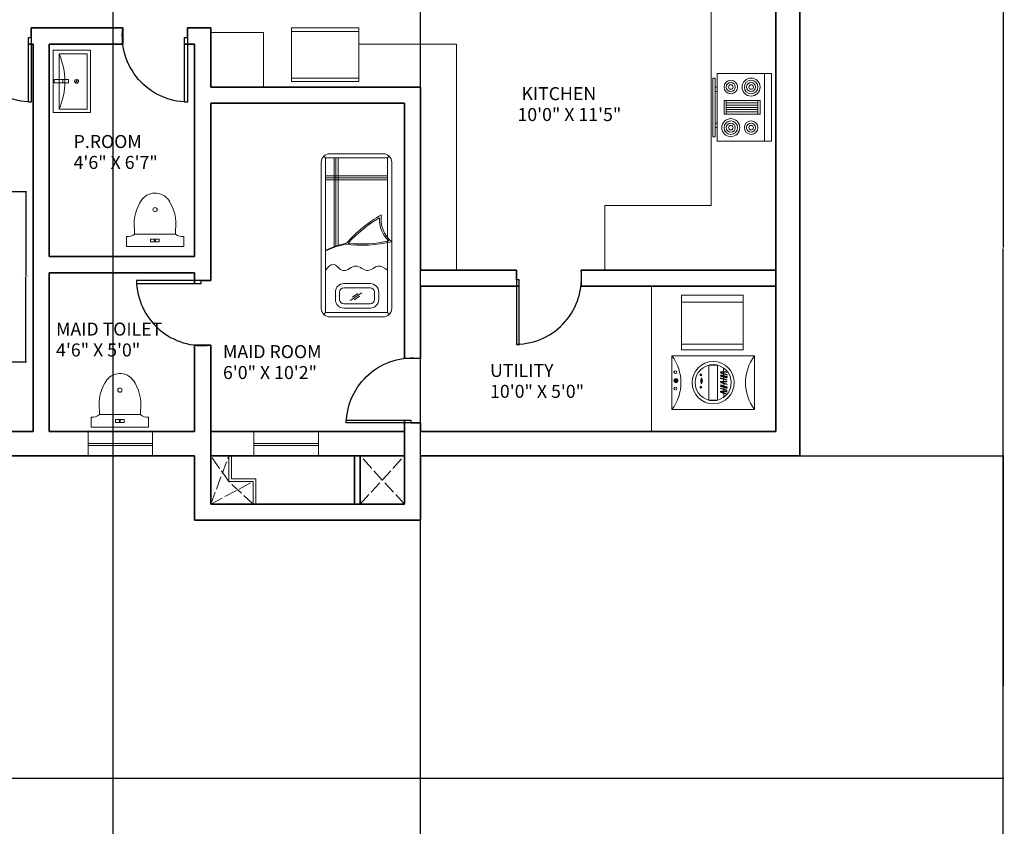
# Model space of a CAD drawing. Units: inches. Extents: x -61 to 1599, y -1316 to 257.
# Tile 195 of 204: x 1233 to 1599, y -579 to -279. Entities that reach past the tile are written whole.
import ezdxf

# ---------------------------------------------------------------- set-up
doc = ezdxf.new("R2010")
doc.units = ezdxf.units.IN
doc.header["$MEASUREMENT"] = 0
doc.linetypes.add('ACAD_ISO02W100', pattern=[15, 12, -3])
for name, color, linetype, lineweight in [('A-ANNO-DIMS', 2, 'Continuous', 18), ('A-AREA-IDEN', 1, 'Continuous', 18), ('A-EQPM', 9, 'Continuous', 18), ('A-FLOR-CASE', 8, 'Continuous', 18), ('A-FLOR-FIXT', 8, 'Continuous', 18), ('A-FLOR-OPEN-HIDN', 8, 'ACAD_ISO02W100', 13), ('A-WALL-JAMB', 4, 'ACAD_ISO02W100', 25), ('DOORS', 2, 'Continuous', 25), ('FURNITURE', 83, 'Continuous', 18), ('WALLS', 4, 'Continuous', 35), ('WINDOWS', 220, 'Continuous', 18)]:
    doc.layers.add(name, color=color, linetype=linetype, lineweight=lineweight)
doc.styles.get("Standard").update_dxf_attribs({"font": 'arial.ttf'})
doc.dimstyles.get("Standard").update_dxf_attribs({"dimtxt": 0.18, "dimasz": 0.18, "dimexe": 0.18, "dimexo": 0.0625, "dimgap": 0.09, "dimtad": 0, "dimtih": 1, "dimtoh": 1, "dimdec": 0, "dimzin": 0, "dimdsep": 46, "dimlunit": 3, "dimtxsty": 'Standard', "dimcen": 0.09, "dimadec": 0, "dimazin": 0, "dimtfac": 1, "dimtdec": 0, "dimtofl": 0, "dimtmove": 0, "dimatfit": 3, "dimfxl": 1, "dimtolj": 1, "dimtzin": 0, "dimarcsym": 0})

# ---------------------------------------------------------------- blocks, each defined once
blk = doc.blocks.new('Range-Oven - 30 in top')
for p, q in [((0, -3), (30, -3)), ((12, -6), (18, -6)), ((13, -20), (13, -6)), ((14, -6), (14, -20)), ((15, -20), (15, -6)), ((16, -6), (16, -20)), ((17, -20), (17, -6)), ((18, -20), (12, -20)), ((6, -24), (6, -25)), ((8, -25), (8, -24)), ((22, -25), (22, -24)), ((24, -24), (24, -25))]:
    blk.add_line(p, q)
for points in [[(0, -24), (0, 0), (30, 0), (30, -24)], [(12, -21), (12, -5), (18, -5), (18, -21)], [(2, -26), (2, -25), (28, -25), (28, -26)]]:
    blk.add_lwpolyline(points, close=True)
for centre, radius in [((6, -9), 4), ((6, -9), 3), ((6, -9), 2), ((6, -9), 1), ((24, -9), 3), ((24, -9), 2), ((24, -9), 1), ((6, -18), 3), ((6, -18), 2), ((6, -18), 1), ((24, -18), 4), ((24, -18), 3), ((24, -18), 2), ((24, -18), 1)]:
    blk.add_circle(centre, radius)
blk = doc.blocks.new('DOOR-SWING-24')
blk.add_line((0, 0), (0, 3.6))
blk.add_lwpolyline([(0, 0), (0, -24), (1.05, -24), (1.05, 0)], close=True)
blk.add_arc((-0.44, 0.62), 24.62, 271.0259, 6.9559)
blk = doc.blocks.new('WIN-24IN')
for p, q in [((0, 4.5), (0, 9)), ((0, 9), (0, 0)), ((24, 9), (24, 0)), ((0, 5.19), (24, 5.19)), ((0, 4.5), (24, 4.5))]:
    blk.add_line(p, q)
blk = doc.blocks.new('WC-FLOOR-MOUNT')
for p, q in [((0, 0), (0, 3.75)), ((3.02, 4.69), (3.02, 6.17)), ((3.02, 4.69), (18.31, 4.69)), ((18.31, 4.69), (18.31, 6.17)), ((21.33, 0), (21.33, 3.75)), ((0, 0), (21.33, 0))]:
    blk.add_line(p, q)
blk.add_lwpolyline([(12.24, 1.73), (8.96, 1.73), (8.96, 2.81), (12.24, 2.81)], close=True)
for centre, radius in [((10.67, 13.73), 0.792), ((10.6, 2.27), 0.208)]:
    blk.add_circle(centre, radius)
for centre, radius, start, end in [((10.67, 13.73), 6.18, 27.6844, 141.4697), ((19.05, 8.26), 16.17, 144.824, 187.4232), ((2.28, 8.26), 16.17, 352.5768, 35.176), ((0.56, 7.25), 3.55, 260.8586, 313.6993), ((20.77, 7.25), 3.55, 226.3007, 279.1414)]:
    blk.add_arc(centre, radius, start, end)
blk = doc.blocks.new('LAVATORY-WALL-2')
blk.add_line((3.67, 10.96), (3.67, 12.19))
for points in [[(0, 23.07), (13.87, 23.07), (13.87, 0), (0, 0)], [(12.66, 21.73), (12.66, 1.19), (2.2, 1.19), (2.2, 21.73)], [(5.78, 12.19), (5.78, 10.96), (0.4, 10.96), (0.4, 12.19)]]:
    blk.add_lwpolyline(points, close=True)
for radius in [0.74, 0.233]:
    blk.add_circle((8.7, 11.57), radius)
blk.add_arc((-20.86, 11.46), 25.25, 335.9939, 24.0061)
blk = doc.blocks.new('WASHING-MACHINE')
for p, q in [((19.24, 4.47), (19.22, 15.41)), ((0.96, 11.16), (1.13, 11)), ((1.49, 11.38), (1.49, 11.15)), ((2.02, 11.15), (1.86, 10.99)), ((11, 9.47), (11, 11.68)), ((0.98, 10.64), (0.75, 10.64)), ((1.12, 10.28), (0.96, 10.12)), ((1.49, 10.12), (1.49, 9.89)), ((1.86, 10.28), (2.02, 10.12)), ((2.23, 10.64), (2, 10.64))]:
    blk.add_line(p, q)
for points in [[(30.68, 0), (0, 0), (0, 19.87), (30.68, 19.87)], [(16.98, 3.42), (13.7, 3.42), (13.7, 16.45), (16.98, 16.45)], [(20.43, 13.78), (18.01, 13.78), (18.01, 13.95), (20.43, 13.95)], [(18.09, 12.45), (20.41, 11.74), (20.35, 11.57), (18.04, 12.29)], [(18.1, 11.71), (20.41, 10.99), (20.36, 10.83), (18.05, 11.54)], [(18.21, 13.64), (20.52, 12.92), (20.47, 12.76), (18.16, 13.47)], [(18.22, 12.89), (20.53, 12.18), (20.48, 12.01), (18.17, 12.73)], [(20.44, 10.23), (18.02, 10.23), (18.02, 10.4), (20.44, 10.4)], [(18.1, 8.63), (20.42, 7.91), (20.37, 7.75), (18.05, 8.46)], [(18.11, 7.88), (20.42, 7.17), (20.37, 7), (18.06, 7.72)], [(18.22, 10.09), (20.53, 9.38), (20.48, 9.21), (18.17, 9.92)], [(18.23, 9.07), (20.54, 8.36), (20.49, 8.19), (18.18, 8.91)], [(20.45, 6.56), (18.03, 6.56), (18.03, 6.73), (20.45, 6.73)], [(18.23, 6.42), (20.54, 5.7), (20.49, 5.54), (18.18, 6.25)]]:
    blk.add_lwpolyline(points, close=True)
for centre, radius in [((15.34, 9.94), 7.85), ((15.34, 9.94), 7.85), ((15.34, 9.94), 6.71), ((1.28, 13.83), 0.526), ((1.49, 10.64), 0.742), ((1.49, 10.64), 0.513), ((10.77, 12.86), 0.381), ((10.77, 12.86), 0.289), ((1.28, 7.75), 0.526), ((1.49, 10.64), 0.178), ((1.49, 10.64), 0.07), ((10.77, 8.29), 0.381), ((10.77, 8.29), 0.289)]:
    blk.add_circle(centre, radius)
for centre, radius, start, end in [((-13.12, 9.94), 16.46, 322.8671, 37.1329), ((43.8, 9.94), 16.46, 142.8671, 217.1329), ((12.8, 10.57), 2.11, 148.4251, 211.5749), ((9.2, 10.57), 2.11, 328.4251, 31.5749)]:
    blk.add_arc(centre, radius, start, end)
blk = doc.blocks.new('UTILITY-CABINET')
for p, q in [((0, 17.69), (23.01, 17.69)), ((0, 2.1), (23.01, 2.1))]:
    blk.add_line(p, q)
blk.add_lwpolyline([(23.01, 0), (0, 0), (0, 20.31), (23.01, 20.31)], close=True)
blk = doc.blocks.new('KITCHEN-BASE-UNIT')
for p, q in [((25.07, 18.6), (0, 18.6)), ((25.07, 1.23), (0, 1.23))]:
    blk.add_line(p, q)
blk.add_lwpolyline([(25.07, 0), (0, 0), (0, 19.92), (25.07, 19.92)], close=True)
blk = doc.blocks.new('*D664')
at = {"layer": 'A-ANNO-DIMS', "color": 0, "lineweight": -2, "transparency": 16777216}
for p, q in [((1225.61, -343.14), (1235.21, -343.14)), ((1235.03, -343.32), (1235.03, -374.58)), ((1235.03, -406.2), (1235.03, -374.95)), ((1225.61, -406.38), (1235.21, -406.38))]:
    blk.add_line(p, q, dxfattribs=at)
at = {"layer": 'A-ANNO-DIMS', "color": 0, "transparency": 16777216}
for points in [[(1235, -343.32), (1235.06, -343.32), (1235.03, -343.14)], [(1235, -406.2), (1235.06, -406.2), (1235.03, -406.38)]]:
    blk.add_solid(points, dxfattribs=at)
at = {"layer": 'DEFPOINTS', "color": 0, "transparency": 16777216}
for p in [(1225.55, -343.14), (1235.03, -343.14), (1225.55, -406.38)]:
    blk.add_point(p, dxfattribs=at)
at = {"layer": 'A-ANNO-DIMS', "color": 0, "transparency": 16777216, "insert": (1235.03, -374.76), "char_height": 0.18, "attachment_point": 5}
blk.add_mtext('\\A1;CONSOLE 63 TYP.', dxfattribs=at)
blk = doc.blocks.new('*D694')
at = {"layer": 'A-ANNO-DIMS', "color": 0, "lineweight": -2, "transparency": 16777216}
for p, q in [((1522.77, -441.32), (1598.48, -441.32)), ((1598.3, -441.5), (1598.3, -526.56)), ((1598.3, -611.99), (1598.3, -526.93)), ((1522.77, -612.17), (1598.48, -612.17))]:
    blk.add_line(p, q, dxfattribs=at)
at = {"layer": 'A-ANNO-DIMS', "color": 0, "transparency": 16777216}
for points in [[(1598.27, -441.5), (1598.33, -441.5), (1598.3, -441.32)], [(1598.27, -611.99), (1598.33, -611.99), (1598.3, -612.17)]]:
    blk.add_solid(points, dxfattribs=at)
at = {"layer": 'DEFPOINTS', "color": 0, "transparency": 16777216}
for p in [(1522.7, -441.32), (1598.3, -441.32), (1522.7, -612.17)]:
    blk.add_point(p, dxfattribs=at)
at = {"layer": 'A-ANNO-DIMS', "color": 0, "transparency": 16777216, "insert": (1598.3, -526.75), "char_height": 0.18, "attachment_point": 5}
blk.add_mtext('\\A1;170.85', dxfattribs=at)
blk = doc.blocks.new('*D698')
at = {"layer": 'A-ANNO-DIMS', "color": 0, "lineweight": -2, "transparency": 16777216}
for p, q in [((644.77, -167.17), (1598.48, -167.17)), ((1598.3, -167.35), (1598.3, -363.99)), ((1598.3, -560.99), (1598.3, -364.35)), ((644.77, -561.17), (1598.48, -561.17))]:
    blk.add_line(p, q, dxfattribs=at)
at = {"layer": 'A-ANNO-DIMS', "color": 0, "transparency": 16777216}
for points in [[(1598.27, -167.35), (1598.33, -167.35), (1598.3, -167.17)], [(1598.27, -560.99), (1598.33, -560.99), (1598.3, -561.17)]]:
    blk.add_solid(points, dxfattribs=at)
at = {"layer": 'DEFPOINTS', "color": 0, "transparency": 16777216}
for p in [(644.7, -167.17), (1598.3, -167.17), (644.7, -561.17)]:
    blk.add_point(p, dxfattribs=at)
at = {"layer": 'A-ANNO-DIMS', "color": 0, "transparency": 16777216, "insert": (1598.3, -364.17), "char_height": 0.18, "attachment_point": 5}
blk.add_mtext('\\A1;394', dxfattribs=at)
blk = doc.blocks.new('*D708')
at = {"layer": 'A-ANNO-DIMS', "color": 0, "lineweight": -2, "transparency": 16777216}
for p, q in [((1267.48, -588.11), (1267.48, 257.46)), ((1267.66, 257.28), (1324.14, 257.28)), ((1381.52, 257.28), (1325.05, 257.28)), ((1381.7, -588.11), (1381.7, 257.46))]:
    blk.add_line(p, q, dxfattribs=at)
at = {"layer": 'A-ANNO-DIMS', "color": 0, "transparency": 16777216}
for points in [[(1267.66, 257.31), (1267.66, 257.25), (1267.48, 257.28)], [(1381.52, 257.31), (1381.52, 257.25), (1381.7, 257.28)]]:
    blk.add_solid(points, dxfattribs=at)
at = {"layer": 'DEFPOINTS', "color": 0, "transparency": 16777216}
for p in [(1381.7, 257.28), (1267.48, -588.17), (1381.7, -588.17)]:
    blk.add_point(p, dxfattribs=at)
at = {"layer": 'A-ANNO-DIMS', "color": 0, "transparency": 16777216, "insert": (1324.59, 257.28), "char_height": 0.18, "attachment_point": 5}
blk.add_mtext('\\A1;114.22', dxfattribs=at)

msp = doc.modelspace()

# ---------------------------------------------------------------- linework, layer by layer
at = {"layer": 'A-FLOR-CASE'}
for p, q in [((1489.7028, -348.3229), (1489.7028, -259.3229)), ((1358.7476, -288.4105), (1395.0519, -288.4105)), ((1395.0519, -288.4105), (1395.0519, -372.3229)), ((1489.7028, -348.3229), (1450.2349, -348.3229)), ((1450.2349, -348.3229), (1450.2349, -372.3229)), ((1467.5747, -432.3229), (1467.5747, -378.3229))]:
    msp.add_line(p, q, dxfattribs=at)
msp.add_lwpolyline([(1323.3268, -304.3229), (1303.7028, -304.3229), (1303.7028, -284.0689), (1323.3268, -284.0689)], close=True, dxfattribs=at)
at = {"layer": 'A-FLOR-OPEN-HIDN', "ltscale": 0.4}
for p, q in [((1303.7028, -459.3229), (1310.4306, -441.3229)), ((1310.4306, -450.9215), (1303.7028, -441.3229)), ((1359.272, -459.3229), (1375.7028, -441.3229)), ((1375.7028, -459.3229), (1359.272, -441.3229)), ((1303.7028, -459.3229), (1319.4965, -450.9215)), ((1319.4965, -459.3229), (1310.4306, -450.9215))]:
    msp.add_line(p, q, dxfattribs=at)
at = {"layer": 'A-FLOR-OPEN-HIDN'}
for p, q in [((1310.4306, -441.3229), (1310.4306, -450.9215)), ((1311.4306, -441.3229), (1311.4306, -449.9215)), ((1311.4306, -449.9215), (1320.4965, -449.9215)), ((1320.4965, -449.9215), (1320.4965, -459.3229)), ((1310.4306, -450.9215), (1319.4965, -450.9215)), ((1319.4965, -450.9215), (1319.4965, -459.3229))]:
    msp.add_line(p, q, dxfattribs=at)
at = {"layer": 'A-WALL-JAMB'}
for p, q in [((1236.999, -282.3229), (1236.999, -288.3229)), ((1271.017, -282.3229), (1271.017, -288.3229)), ((1295.017, -282.3229), (1295.017, -288.3229)), ((1417.3522, -372.3229), (1417.3522, -378.3229)), ((1441.3522, -372.3229), (1441.3522, -378.3229)), ((1303.7028, -376.2211), (1297.7028, -376.2211)), ((1303.7028, -400.2211), (1297.7028, -400.2211)), ((1381.7028, -405.1414), (1375.7028, -405.1458)), ((1381.7028, -429.1414), (1375.7028, -429.1414))]:
    msp.add_line(p, q, dxfattribs=at)
at = {"layer": 'FURNITURE'}
for p, q in [((1346.3698, -330.6674), (1345.7148, -330.0124)), ((1349.5985, -363.6544), (1349.5985, -330.6674)), ((1350.1865, -363.443), (1350.1865, -330.6674)), ((1351.0588, -363.1542), (1351.0588, -330.6674)), ((1369.4076, -330.6674), (1370.0626, -330.0124)), ((1369.4076, -337.3084), (1346.3698, -337.3084)), ((1369.4076, -338.0177), (1346.3698, -338.0177)), ((1369.4076, -338.7871), (1346.3698, -338.7871)), ((1359.8729, -380.7881), (1355.5662, -383.6749)), ((1356.3763, -382.3874), (1358.413, -381.0304)), ((1357.072, -383.4316), (1359.1087, -382.0746)), ((1346.3698, -388.1313), (1345.7148, -388.7863)), ((1370.0626, -388.7863), (1369.4076, -388.1313))]:
    msp.add_line(p, q, dxfattribs=at)
for points in [[(1347.9511, -329.0861), (1367.8263, -329.0861, -0.41421356), (1370.989, -332.2487), (1370.989, -386.55, -0.41421356), (1367.8263, -389.7126), (1347.9511, -389.7126, -0.41421356), (1344.7885, -386.55), (1344.7885, -332.2487, -0.41421356)], [(1353.197, -377.3355), (1362.9839, -377.3355, -0.41421356), (1366.1465, -380.4982), (1366.1465, -383.3141, -0.41421356), (1362.9839, -386.4767), (1353.197, -386.4767, -0.41421356), (1350.0344, -383.3141), (1350.0344, -380.4982, -0.41421356)], [(1353.197, -378.9168), (1362.9839, -378.9168, -0.41421356), (1364.5652, -380.4982), (1364.5652, -383.3141, -0.41421356), (1362.9839, -384.8954), (1353.197, -384.8954, -0.41421356), (1351.6157, -383.3141), (1351.6157, -380.4982, -0.41421356)]]:
    msp.add_lwpolyline(points, format="xyb", close=True, dxfattribs=at)
msp.add_lwpolyline([(1346.3698, -330.6674), (1369.4076, -330.6674), (1369.4076, -388.1313), (1346.3698, -388.1313)], close=True, dxfattribs=at)
for centre, radius, start, end in [((1390.8702, -394.1626), 48.5558, 119.302799, 139.065497), ((1390.7906, -394.9259), 48.5558, 120.122754, 137.951503), ((1377.4118, -353.4771), 11.0029, 177.136894, 226.788842), ((1378.0028, -353.343), 11.0029, 172.042189, 230.397858), ((1359.953, -314.5357), 48.5558, 262.813151, 283.137248), ((1359.4332, -314.0773), 48.5558, 264.446321, 282.422187), ((1360.2263, -392.3018), 30.5553, 101.397161, 116.967867), ((1359.9164, -392.6627), 30.5553, 101.397161, 116.317614)]:
    msp.add_arc(centre, radius, start, end, dxfattribs=at)
msp.add_open_spline([(1369.4076, -372.395), (1368.2379, -371.5093), (1365.818, -369.677), (1361.9669, -374.1451), (1357.6119, -368.943), (1353.0321, -374.5225), (1349.3585, -368.6867), (1347.2784, -371.2237), (1346.3698, -372.3318)], degree=3, knots=[0, 0, 0, 0, 3.84254534, 7.94890144, 12.81558195, 17.74158221, 22.25649, 25.75782552, 25.75782552, 25.75782552, 25.75782552], dxfattribs=at)
at = {"layer": 'WALLS'}
for p, q in [((1522.7028, -441.3229), (1522.7028, -67.169)), ((1513.7028, -282.3229), (1513.7028, -175.3229)), ((1236.999, -282.3229), (1271.017, -282.3229)), ((1295.017, -282.3229), (1303.7028, -282.3229)), ((1303.7028, -282.3229), (1303.7028, -304.3229)), ((1513.7028, -282.3229), (1513.7028, -378.3229)), ((1235.949, -288.3229), (1237.7028, -288.3229)), ((1237.7028, -288.3229), (1237.7028, -432.3229)), ((1243.7028, -288.3229), (1243.7028, -367.3229)), ((1243.7028, -288.3229), (1271.0214, -288.3229)), ((1293.967, -288.3229), (1297.7028, -288.3229)), ((1297.7028, -288.3229), (1297.7028, -367.3229)), ((1303.7028, -304.3229), (1381.7028, -304.3229)), ((1381.7028, -304.3229), (1381.7028, -372.3229)), ((1303.7028, -310.3229), (1303.7028, -376.2211)), ((1303.7028, -310.3229), (1375.7028, -310.3229)), ((1375.7028, -310.3229), (1375.7028, -405.1458)), ((1243.7028, -367.3229), (1297.7028, -367.3229)), ((1381.7028, -372.3229), (1417.3522, -372.3229)), ((1441.3522, -372.3229), (1513.7028, -372.3229)), ((1243.7028, -373.3229), (1243.7028, -432.3229)), ((1243.7028, -373.3229), (1297.7028, -373.3229)), ((1297.7028, -373.3229), (1297.7028, -377.2711)), ((1381.7028, -378.3229), (1381.7028, -405.1414)), ((1381.7028, -378.3229), (1418.4022, -378.3229)), ((1441.3477, -378.3229), (1513.7028, -378.3229)), ((1513.7028, -432.3229), (1513.7028, -378.3229)), ((1297.7028, -400.2167), (1297.7028, -432.3229)), ((1303.7028, -400.2211), (1303.7028, -441.3229)), ((1375.7028, -428.0914), (1375.7028, -441.3229)), ((1381.7028, -429.1414), (1381.7028, -432.3229)), ((1215.7028, -432.3229), (1237.7028, -432.3229)), ((1243.7028, -432.3229), (1297.7028, -432.3229)), ((1303.7028, -432.3229), (1305.7028, -432.3229)), ((1305.7028, -432.3229), (1375.7028, -432.3229)), ((1381.7028, -432.3229), (1513.7028, -432.3229)), ((1215.7028, -441.3229), (1297.7028, -441.3229)), ((1297.7028, -441.3229), (1297.7028, -465.3229)), ((1303.7028, -441.3229), (1305.7028, -441.3229)), ((1303.7028, -441.3229), (1303.7028, -459.3229)), ((1305.7028, -441.3229), (1375.7028, -441.3229)), ((1357.1436, -459.3229), (1357.1436, -441.3229)), ((1359.272, -459.3229), (1359.272, -441.3229)), ((1375.7028, -441.3229), (1375.7028, -459.3229)), ((1381.7028, -441.3229), (1522.7028, -441.3229)), ((1381.7028, -441.3229), (1381.7028, -465.3229)), ((1375.7028, -459.3229), (1303.7028, -459.3229)), ((1381.7028, -465.3229), (1297.7028, -465.3229))]:
    msp.add_line(p, q, dxfattribs=at)

# ---------------------------------------------------------------- block references
at = {"layer": 'A-EQPM', "xscale": 0.8378013827109642, "yscale": 0.8378013827109642, "zscale": 0.8378013827109642, "rotation": 270}
msp.add_blockref('Range-Oven - 30 in top', (1512.1022, -299.295), dxfattribs=at)
at = {"layer": 'A-EQPM'}
msp.add_blockref('WASHING-MACHINE', (1475.133, -424.099), dxfattribs=at)
at = {"layer": 'A-FLOR-CASE'}
for name, p in [('KITCHEN-BASE-UNIT', (1333.674, -302.245)), ('UTILITY-CABINET', (1478.634, -401.916))]:
    msp.add_blockref(name, p, dxfattribs=at)
at = {"layer": 'A-FLOR-FIXT'}
for name, p in [('LAVATORY-WALL-2', (1245.1172, -313.7295)), ('WC-FLOOR-MOUNT', (1272.349, -363.6106)), ('WC-FLOOR-MOUNT', (1259.2982, -430.6752))]:
    msp.add_blockref(name, p, dxfattribs=at)
at = {"layer": 'DOORS', "extrusion": (0, 0, -1), "zscale": -1}
for p in [(-1236.999, -285.9229), (-1295.017, -285.9229)]:
    msp.add_blockref('DOOR-SWING-24', p, dxfattribs=at)
at = {"layer": 'DOORS'}
msp.add_blockref('DOOR-SWING-24', (1417.3522, -375.9229), dxfattribs=at)
at = {"layer": 'DOORS', "rotation": 270.0000000000009}
msp.add_blockref('DOOR-SWING-24', (1300.1028, -376.2211), dxfattribs=at)
at = {"layer": 'DOORS', "extrusion": (0, 0, -1), "zscale": -1, "rotation": 90.00000000000087}
msp.add_blockref('DOOR-SWING-24', (-1378.1028, -429.1414), dxfattribs=at)
at = {"layer": 'WINDOWS', "rotation": 180}
for p in [(1282.1139, -432.3228), (1343.7033, -432.3228)]:
    msp.add_blockref('WIN-24IN', p, dxfattribs=at)

# ---------------------------------------------------------------- texts
at = {"layer": 'A-AREA-IDEN'}
for s, height, p in [(' KITCHEN', 4.8321, (1417.7144, -309.1831)), ('10\'0" X 11\'5"', 4.832098, (1417.7144, -316.9454)), ('P.ROOM', 4.8321, (1252.7407, -326.9772)), ('4\'6" X 6\'7"', 4.832098, (1252.7407, -334.7395)), ('MAID TOILET', 4.832098, (1246.2172, -396.6681)), ('4\'6" X 5\'0"', 4.832098, (1246.2172, -404.4305)), ('MAID ROOM', 4.8321, (1308.2598, -405.0558)), ('6\'0" X 10\'2"', 4.832098, (1308.2598, -412.8182)), ('UTILITY', 4.8321, (1407.5332, -412.0454)), ('10\'0" X 5\'0"', 4.832098, (1407.5332, -419.8078))]:
    msp.add_text(s, height=height, dxfattribs=at).set_placement(p)

# ---------------------------------------------------------------- dimensions: what is measured, and where the dimension line sits
at = {"layer": 'A-ANNO-DIMS'}
dim = msp.add_linear_dim(base=(1381.7028, 257.2771), p1=(1267.4807, -588.169), p2=(1381.7028, -588.169), dimstyle='Standard', override={"dimdec": 2, "dimlfac": 1, "dimrnd": 0, "dimzin": 0, "dimdsep": 46, "dimlunit": 2}, dxfattribs=at)
dim.commit()
dim.dimension.update_dxf_attribs({"geometry": '*D708', "text_midpoint": (1324.5917, 257.2771)})
for base, p1, p2, override, picture, middle in [((1598.3028, -167.169), (644.7028, -561.169), (644.7028, -167.169), {"dimdec": 0, "dimlfac": 1, "dimrnd": 0, "dimzin": 0, "dimdsep": 46, "dimlunit": 2}, '*D698', (1598.3028, -364.169)), ((1598.3028, -441.3229), (1522.7028, -612.169), (1522.7028, -441.3229), {"dimdec": 2, "dimlfac": 1, "dimrnd": 0, "dimzin": 0, "dimdsep": 46, "dimlunit": 2}, '*D694', (1598.3028, -526.746))]:
    dim = msp.add_linear_dim(base=base, p1=p1, p2=p2, angle=90, dimstyle='Standard', override=override, dxfattribs=at)
    dim.commit()
    dim.dimension.update_dxf_attribs({"geometry": picture, "text_midpoint": middle})
dim = msp.add_linear_dim(base=(1235.0311, -343.1432), p1=(1225.5451, -406.3834), p2=(1225.5451, -343.1432), angle=90, text='CONSOLE <> TYP.', dimstyle='Standard', override={"dimdec": 0, "dimlfac": 1, "dimrnd": 0, "dimzin": 0, "dimdsep": 46, "dimlunit": 2}, dxfattribs=at)
dim.commit()
dim.dimension.update_dxf_attribs({"geometry": '*D664', "text_midpoint": (1235.0311, -374.7633)})

doc.saveas('drawing.dxf')
